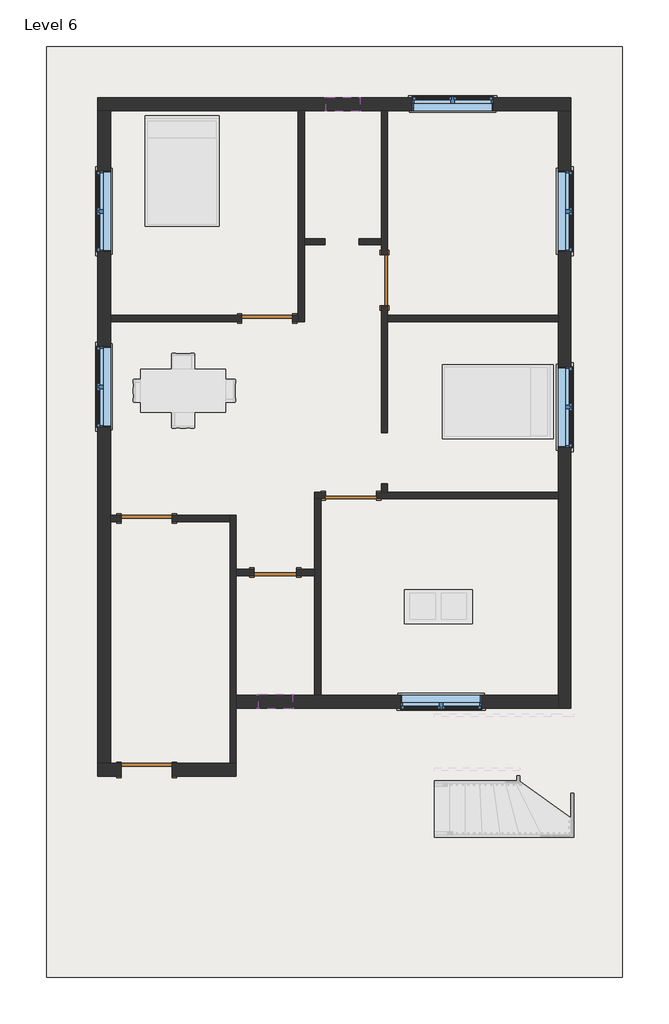
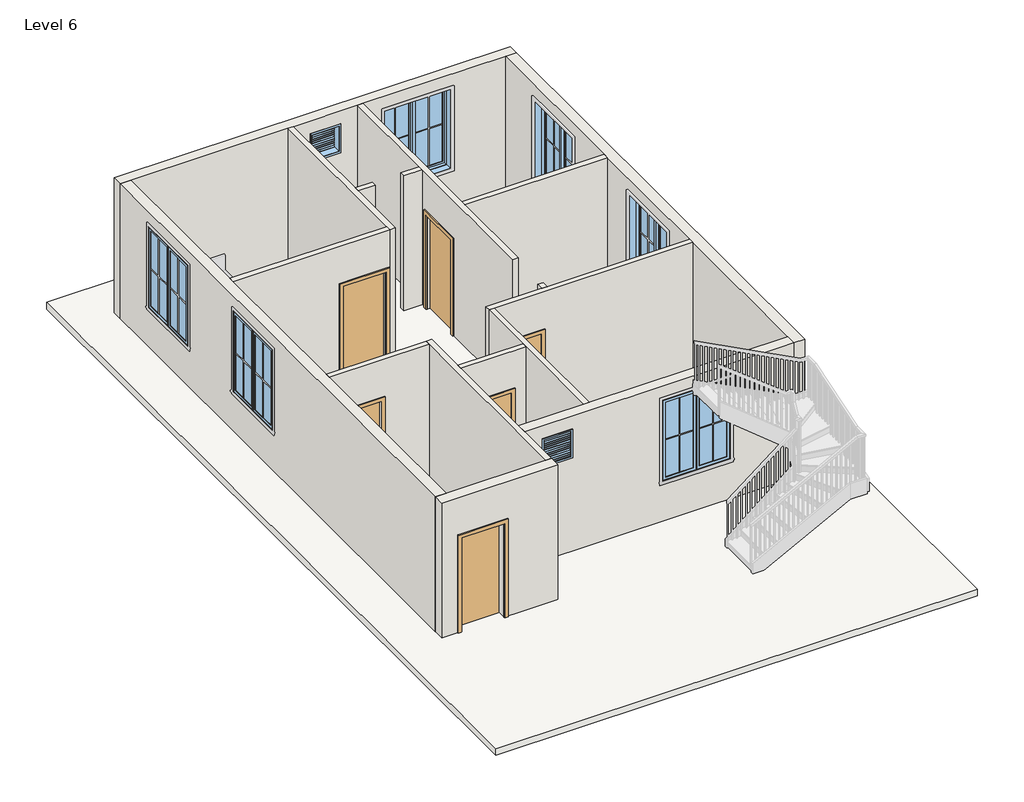
# One storey, part 1 of 3: 17 walls, 8 windows, 6 doors, 1 roof.
"""IFC4 building model written with IfcOpenShell, lengths in millimetres."""

from ifc_helpers import new_model, si_unit, frame, origin, place, context, project, spatial, polyline, outline, extrude, faceted_brep, transform, mapped, element, save
from components import door_214872d5, single_flush_door_3_e5f9f3c4, single_flush_door_3_305aa2a5, single_flush_door_3_a90ba1ad, window_9ac97e1a, window_f2d8fef0

model = new_model("IFC4")

# Units and contexts
model_context = context("Model", 3, world=origin())
ifc_project = project(units=[si_unit("LENGTHUNIT", "METRE", prefix="MILLI")], contexts=[model_context])

# Site, building, storey
site = spatial("IfcSite", under=ifc_project)
building = spatial("IfcBuilding", under=site)
storey = spatial("IfcBuildingStorey", under=building, Name="Level 6", Elevation=12801.6)

# Doors
placement = place(None, origin())
door_shape = door_214872d5(model_context)
element("IfcDoor", 1, ObjectType="Single-Flush : DOOR 2'6\"", at=placement, inside=storey, context=model_context, shape_type="MappedRepresentation", body=[
    mapped(door_shape, transform((-2309.3144966, -2885.2590409, 12801.6), x_axis=(-1.0, 0.0, 0.0), y_axis=(0.0, -1.0, 0.0), z_axis=(0.0, 0.0, 1.0))),
])
single_flush_door_3_shape = single_flush_door_3_e5f9f3c4(model_context)
element("IfcDoor", 2, ObjectType="Single-Flush : DOOR 3'", at=placement, inside=storey, context=model_context, shape_type="MappedRepresentation", body=[
    mapped(single_flush_door_3_shape, transform((-2455.3644966, 1648.6409591, 12801.6), x_axis=(1.0, 0.0, 0.0), y_axis=(0.0, 1.0, 0.0), z_axis=(0.0, 0.0, 1.0))),
])
element("IfcDoor", 3, ObjectType="Single-Flush : DOOR 3'", at=placement, inside=storey, context=model_context, shape_type="MappedRepresentation", body=[
    mapped(single_flush_door_3_shape, transform((-359.8644966, 2334.4409591, 12801.6), x_axis=(0.0, -1.0, 0.0), y_axis=(1.0, 0.0, 0.0), z_axis=(0.0, 0.0, 1.0))),
])
element("IfcDoor", 4, ObjectType="Single-Flush : DOOR 3'", at=placement, inside=storey, context=model_context, shape_type="MappedRepresentation", body=[
    mapped(single_flush_door_3_shape, transform((-956.7644966, -1513.6590409, 12801.6), x_axis=(-1.0, 0.0, 0.0), y_axis=(0.0, -1.0, 0.0), z_axis=(0.0, 0.0, 1.0))),
])
single_flush_door_3_2_shape = single_flush_door_3_305aa2a5(model_context)
element("IfcDoor", 5, ObjectType="Single-Flush : DOOR 3'", at=placement, inside=storey, context=model_context, shape_type="MappedRepresentation", body=[
    mapped(single_flush_door_3_2_shape, transform((-4608.0144966, -1920.0590409, 12801.6), x_axis=(-1.0, 0.0, 0.0), y_axis=(0.0, -1.0, 0.0), z_axis=(0.0, 0.0, 1.0))),
])
single_flush_door_3_3_shape = single_flush_door_3_a90ba1ad(model_context)
element("IfcDoor", 6, ObjectType="Single-Flush : DOOR 3'", at=placement, inside=storey, context=model_context, shape_type="MappedRepresentation", body=[
    mapped(single_flush_door_3_3_shape, transform((-4608.0144966, -6409.5090409, 12801.6), x_axis=(-1.0, 0.0, 0.0), y_axis=(0.0, -1.0, 0.0), z_axis=(0.0, 0.0, 1.0))),
])

# Roof
element("IfcRoof", 7, ObjectType="ROOF 6\"", at=placement, inside=storey, context=model_context, shape_type="SweptSolid", body=[
    extrude(outline(polyline([(-6398.7144966, 6506.3909591), (3888.2855034, 6506.3909591), (3888.2855034, -10115.6142473), (-6398.7144966, -10115.6142473), (-6398.7144966, 6506.3909591)])), frame((0.0, 0.0, 12649.2), z_axis=(0.0, 0.0, 1.0), x_axis=(1.0, 0.0, 0.0)), (0.0, 0.0, 1.0), 152.4),
])

# Walls
element("IfcWall", 8, ObjectType="WALL 4.5\"", at=placement, inside=storey, context=model_context, shape_type="Brep", body=[
    faceted_brep([(-1902.9144966, 5363.3909591, 12801.6), (-1902.9144966, 1705.7909591, 12801.6), (-1902.9144966, 1591.4909591, 12801.6), (-1902.9144966, 1591.4909591, 15849.6), (-1902.9144966, 1705.7909591, 15849.6), (-1902.9144966, 5363.3909591, 15849.6), (-1788.6144966, 5363.3909591, 12801.6), (-1788.6144966, 5363.3909591, 15849.6), (-1788.6144966, 3077.3909591, 15849.6), (-1788.6144966, 2963.0909591, 15849.6), (-1788.6144966, 1591.4909591, 15849.6), (-1788.6144966, 1591.4909591, 12801.6), (-1788.6144966, 2963.0909591, 12801.6), (-1788.6144966, 3077.3909591, 12801.6)], [[[0, 1, 2, 3, 4, 5]], [[6, 7, 8, 9, 10, 11, 12, 13]], [[2, 1, 0, 6, 13, 12, 11]], [[0, 5, 7, 6]], [[3, 2, 11, 10]], [[5, 4, 3, 10, 9, 8, 7]]]),
])
element("IfcWall", 9, ObjectType="WALL 4.5\"", at=placement, inside=storey, context=model_context, shape_type="SweptSolid", body=[
    extrude(outline(polyline([(14935.2, -1998.1644966), (12801.6, -1998.1644966), (12801.6, -1902.9144966), (15849.6, -1902.9144966), (15849.6, -5255.7144966), (12801.6, -5255.7144966), (12801.6, -2912.5644966), (14935.2, -2912.5644966), (14935.2, -1998.1644966)])), frame((0.0, 1591.4909591, 0.0), z_axis=(0.0, 1.0, 0.0), x_axis=(0.0, 0.0, 1.0)), (0.0, 0.0, 1.0), 114.3),
])
element("IfcWall", 10, ObjectType="WALL 4.5\"", at=placement, inside=storey, context=model_context, shape_type="Brep", body=[
    faceted_brep([(-417.0144966, 1877.2409591, 14935.2), (-417.0144966, 1877.2409591, 12801.6), (-417.0144966, -389.7090409, 12801.6), (-417.0144966, -389.7090409, 15849.6), (-417.0144966, 2963.0909591, 15849.6), (-417.0144966, 3077.3909591, 15849.6), (-417.0144966, 5363.3909591, 15849.6), (-417.0144966, 5363.3909591, 12801.6), (-417.0144966, 3077.3909591, 12801.6), (-417.0144966, 2963.0909591, 12801.6), (-417.0144966, 2791.6409591, 12801.6), (-417.0144966, 2791.6409591, 14935.2), (-302.7144966, -389.7090409, 12801.6), (-302.7144966, 1591.4909591, 12801.6), (-302.7144966, 1705.7909591, 12801.6), (-302.7144966, 1877.2409591, 12801.6), (-302.7144966, 1877.2409591, 14935.2), (-302.7144966, 2791.6409591, 14935.2), (-302.7144966, 2791.6409591, 12801.6), (-302.7144966, 5363.3909591, 12801.6), (-302.7144966, 5363.3909591, 15849.6), (-302.7144966, 1705.7909591, 15849.6), (-302.7144966, 1591.4909591, 15849.6), (-302.7144966, -389.7090409, 15849.6)], [[[0, 1, 2, 3, 4, 5, 6, 7, 8, 9, 10, 11]], [[12, 13, 14, 15, 16, 17, 18, 19, 20, 21, 22, 23]], [[2, 1, 15, 14, 13, 12]], [[10, 9, 8, 7, 19, 18]], [[3, 2, 12, 23]], [[7, 6, 20, 19]], [[16, 15, 1, 0]], [[17, 16, 0, 11]], [[18, 17, 11, 10]], [[6, 5, 4, 3, 23, 22, 21, 20]]]),
])
element("IfcWall", 11, ObjectType="WALL 4.5\"", at=placement, inside=storey, context=model_context, shape_type="SweptSolid", body=[
    extrude(outline(polyline([(-302.7144966, 1705.7909591), (2745.2855034, 1705.7909591), (2745.2855034, 1591.4909591), (-302.7144966, 1591.4909591), (-302.7144966, 1705.7909591)])), frame((0.0, 0.0, 12801.6), z_axis=(0.0, 0.0, 1.0), x_axis=(1.0, 0.0, 0.0)), (0.0, 0.0, 1.0), 3048.0),
])
element("IfcWall", 12, ObjectType="WALL 4.5\"", at=placement, inside=storey, context=model_context, shape_type="SweptSolid", body=[
    extrude(outline(polyline([(-1423.1234474, 2963.0909591), (-1788.6144966, 2963.0909591), (-1788.6144966, 3077.3909591), (-1423.1234474, 3077.3909591), (-1423.1234474, 2963.0909591)])), frame((0.0, 0.0, 12801.6), z_axis=(0.0, 0.0, 1.0), x_axis=(1.0, 0.0, 0.0)), (0.0, 0.0, 1.0), 3048.0),
])
element("IfcWall", 13, ObjectType="WALL 4.5\"", at=placement, inside=storey, context=model_context, shape_type="Brep", body=[
    faceted_brep([(-1413.9644966, -1456.5090409, 14935.2), (-1413.9644966, -1456.5090409, 12801.6), (-1610.8144966, -1456.5090409, 12801.6), (-1610.8144966, -1456.5090409, 15849.6), (-417.0144966, -1456.5090409, 15849.6), (-302.7144966, -1456.5090409, 15849.6), (2745.2855034, -1456.5090409, 15849.6), (2745.2855034, -1456.5090409, 12801.6), (-302.7144966, -1456.5090409, 12801.6), (-417.0144966, -1456.5090409, 12801.6), (-499.5644966, -1456.5090409, 12801.6), (-499.5644966, -1456.5090409, 14935.2), (-1610.8144966, -1570.8090409, 12801.6), (-1496.5144966, -1570.8090409, 12801.6), (-1413.9644966, -1570.8090409, 12801.6), (-1413.9644966, -1570.8090409, 14935.2), (-499.5644966, -1570.8090409, 14935.2), (-499.5644966, -1570.8090409, 12801.6), (2745.2855034, -1570.8090409, 12801.6), (2745.2855034, -1570.8090409, 15849.6), (-1496.5144966, -1570.8090409, 15849.6), (-1610.8144966, -1570.8090409, 15849.6)], [[[0, 1, 2, 3, 4, 5, 6, 7, 8, 9, 10, 11]], [[12, 13, 14, 15, 16, 17, 18, 19, 20, 21]], [[2, 1, 14, 13, 12]], [[10, 9, 8, 7, 18, 17]], [[7, 6, 19, 18]], [[3, 2, 12, 21]], [[15, 14, 1, 0]], [[16, 15, 0, 11]], [[17, 16, 11, 10]], [[6, 5, 4, 3, 21, 20, 19]]]),
])
element("IfcWall", 14, ObjectType="WALL 4.5\"", at=placement, inside=storey, context=model_context, shape_type="SweptSolid", body=[
    extrude(outline(polyline([(-302.7144966, -1304.1090409), (-302.7144966, -1456.5090409), (-417.0144966, -1456.5090409), (-417.0144966, -1304.1090409), (-302.7144966, -1304.1090409)])), frame((0.0, 0.0, 12801.6), z_axis=(0.0, 0.0, 1.0), x_axis=(1.0, 0.0, 0.0)), (0.0, 0.0, 1.0), 3048.0),
])
element("IfcWall", 15, ObjectType="WALL 4.5\"", at=placement, inside=storey, context=model_context, shape_type="Brep", body=[
    faceted_brep([(-1610.8144966, -1570.8090409, 12801.6), (-1610.8144966, -2828.1090409, 12801.6), (-1610.8144966, -2942.4090409, 12801.6), (-1610.8144966, -5076.0090409, 12801.6), (-1610.8144966, -5076.0090409, 15849.6), (-1610.8144966, -2942.4090409, 15849.6), (-1610.8144966, -2828.1090409, 15849.6), (-1610.8144966, -1570.8090409, 15849.6), (-1496.5144966, -1570.8090409, 12801.6), (-1496.5144966, -1570.8090409, 15849.6), (-1496.5144966, -5076.0090409, 15849.6), (-1496.5144966, -5076.0090409, 12801.6)], [[[0, 1, 2, 3, 4, 5, 6, 7]], [[8, 9, 10, 11]], [[3, 2, 1, 0, 8, 11]], [[0, 7, 9, 8]], [[4, 3, 11, 10]], [[7, 6, 5, 4, 10, 9]]]),
])
element("IfcWall", 16, ObjectType="WALL 4.5\"", at=placement, inside=storey, context=model_context, shape_type="SweptSolid", body=[
    extrude(outline(polyline([(12801.6, -3007.8144966), (12801.6, -2690.3144966), (14935.2, -2690.3144966), (14935.2, -1928.3144966), (12801.6, -1928.3144966), (12801.6, -1610.8144966), (15849.6, -1610.8144966), (15849.6, -3007.8144966), (12801.6, -3007.8144966)])), frame((0.0, -2942.4090409, 0.0), z_axis=(0.0, 1.0, 0.0), x_axis=(0.0, 0.0, 1.0)), (0.0, 0.0, 1.0), 114.3),
])
element("IfcWall", 17, ObjectType="WALL 4.5\"", at=placement, inside=storey, context=model_context, shape_type="Brep", body=[
    faceted_brep([(-3007.8144966, -6295.2090409, 12801.6), (-3007.8144966, -5304.6090409, 12801.6), (-3007.8144966, -5076.0090409, 12801.6), (-3007.8144966, -2942.4090409, 12801.6), (-3007.8144966, -2828.1090409, 12801.6), (-3007.8144966, -1862.9090409, 12801.6), (-3007.8144966, -1862.9090409, 15849.6), (-3007.8144966, -2828.1090409, 15849.6), (-3007.8144966, -2942.4090409, 15849.6), (-3007.8144966, -5076.0090409, 15849.6), (-3007.8144966, -5304.6090409, 15849.6), (-3007.8144966, -6295.2090409, 15849.6), (-3122.1144966, -6295.2090409, 12801.6), (-3122.1144966, -6295.2090409, 15849.6), (-3122.1144966, -1977.2090409, 15849.6), (-3122.1144966, -1862.9090409, 15849.6), (-3122.1144966, -1862.9090409, 12801.6), (-3122.1144966, -1977.2090409, 12801.6)], [[[0, 1, 2, 3, 4, 5, 6, 7, 8, 9, 10, 11]], [[12, 13, 14, 15, 16, 17]], [[5, 4, 3, 2, 1, 0, 12, 17, 16]], [[0, 11, 13, 12]], [[6, 5, 16, 15]], [[11, 10, 9, 8, 7, 6, 15, 14, 13]]]),
])
element("IfcWall", 18, ObjectType="WALL 4.5\"", at=placement, inside=storey, context=model_context, shape_type="SweptSolid", body=[
    extrude(outline(polyline([(12801.6, -5255.7144966), (12801.6, -5065.2144966), (14935.2, -5065.2144966), (14935.2, -4150.8144966), (12801.6, -4150.8144966), (12801.6, -3122.1144966), (15849.6, -3122.1144966), (15849.6, -5255.7144966), (12801.6, -5255.7144966)])), frame((0.0, -1977.2090409, 0.0), z_axis=(0.0, 1.0, 0.0), x_axis=(0.0, 0.0, 1.0)), (0.0, 0.0, 1.0), 114.3),
])
element("IfcWall", 19, ObjectType="WALL 4.5\"", at=placement, inside=storey, context=model_context, shape_type="SweptSolid", body=[
    extrude(outline(polyline([(-417.0144966, 2963.0909591), (-814.3659123, 2963.0909591), (-814.3659123, 3077.3909591), (-417.0144966, 3077.3909591), (-417.0144966, 2963.0909591)])), frame((0.0, 0.0, 12801.6), z_axis=(0.0, 0.0, 1.0), x_axis=(1.0, 0.0, 0.0)), (0.0, 0.0, 1.0), 3048.0),
])
element("IfcWall", 20, ObjectType="WALL 9\"", at=placement, inside=storey, context=model_context, shape_type="Brep", body=[
    faceted_brep([(-5484.3144966, 5363.3909591, 12801.6), (-5255.7144966, 5363.3909591, 12801.6), (-1902.9144966, 5363.3909591, 12801.6), (-1788.6144966, 5363.3909591, 12801.6), (-417.0144966, 5363.3909591, 12801.6), (-302.7144966, 5363.3909591, 12801.6), (2745.2855034, 5363.3909591, 12801.6), (2973.8855034, 5363.3909591, 12801.6), (2973.8855034, 5363.3909591, 15849.6), (2745.2855034, 5363.3909591, 15849.6), (-302.7144966, 5363.3909591, 15849.6), (-417.0144966, 5363.3909591, 15849.6), (-1788.6144966, 5363.3909591, 15849.6), (-1902.9144966, 5363.3909591, 15849.6), (-5255.7144966, 5363.3909591, 15849.6), (-5484.3144966, 5363.3909591, 15849.6), (1583.2355034, 5363.3909591, 15544.8), (1583.2355034, 5363.3909591, 13716.0), (135.4355034, 5363.3909591, 13716.0), (135.4355034, 5363.3909591, 15544.8), (-1407.6144966, 5363.3909591, 15544.8), (-798.0144966, 5363.3909591, 15544.8), (-798.0144966, 5363.3909591, 14935.2), (-1407.6144966, 5363.3909591, 14935.2), (-5484.3144966, 5591.9909591, 12801.6), (-5484.3144966, 5591.9909591, 15849.6), (2973.8855034, 5591.9909591, 15849.6), (2973.8855034, 5591.9909591, 12801.6), (1583.2355034, 5591.9909591, 15544.8), (135.4355034, 5591.9909591, 15544.8), (135.4355034, 5591.9909591, 13716.0), (1583.2355034, 5591.9909591, 13716.0), (-1407.6144966, 5591.9909591, 15544.8), (-1407.6144966, 5591.9909591, 14935.2), (-798.0144966, 5591.9909591, 14935.2), (-798.0144966, 5591.9909591, 15544.8)], [[[0, 1, 2, 3, 4, 5, 6, 7, 8, 9, 10, 11, 12, 13, 14, 15], [16, 17, 18, 19], [20, 21, 22, 23]], [[24, 25, 26, 27], [28, 29, 30, 31], [32, 33, 34, 35]], [[7, 6, 5, 4, 3, 2, 1, 0, 24, 27]], [[8, 7, 27, 26]], [[0, 15, 25, 24]], [[17, 16, 28, 31]], [[18, 17, 31, 30]], [[19, 18, 30, 29]], [[16, 19, 29, 28]], [[33, 32, 20, 23]], [[34, 33, 23, 22]], [[35, 34, 22, 21]], [[32, 35, 21, 20]], [[15, 14, 13, 12, 11, 10, 9, 8, 26, 25]]]),
])
element("IfcWall", 21, ObjectType="WALL 9\"", at=placement, inside=storey, context=model_context, shape_type="Brep", body=[
    faceted_brep([(2745.2855034, 5363.3909591, 12801.6), (2745.2855034, 1705.7909591, 12801.6), (2745.2855034, 1591.4909591, 12801.6), (2745.2855034, -1456.5090409, 12801.6), (2745.2855034, -1570.8090409, 12801.6), (2745.2855034, -5076.0090409, 12801.6), (2745.2855034, -5304.6090409, 12801.6), (2745.2855034, -5304.6090409, 15849.6), (2745.2855034, -5076.0090409, 15849.6), (2745.2855034, -1570.8090409, 15849.6), (2745.2855034, -1456.5090409, 15849.6), (2745.2855034, 1591.4909591, 15849.6), (2745.2855034, 1705.7909591, 15849.6), (2745.2855034, 5363.3909591, 15849.6), (2745.2855034, -656.4090409, 15544.8), (2745.2855034, -656.4090409, 13716.0), (2745.2855034, 791.3909591, 13716.0), (2745.2855034, 791.3909591, 15544.8), (2745.2855034, 2839.2659591, 15544.8), (2745.2855034, 2839.2659591, 13716.0), (2745.2855034, 4287.0659591, 13716.0), (2745.2855034, 4287.0659591, 15544.8), (2973.8855034, 5363.3909591, 12801.6), (2973.8855034, 5363.3909591, 15849.6), (2973.8855034, -5304.6090409, 15849.6), (2973.8855034, -5304.6090409, 12801.6), (2973.8855034, -656.4090409, 15544.8), (2973.8855034, 791.3909591, 15544.8), (2973.8855034, 791.3909591, 13716.0), (2973.8855034, -656.4090409, 13716.0), (2973.8855034, 2839.2659591, 15544.8), (2973.8855034, 4287.0659591, 15544.8), (2973.8855034, 4287.0659591, 13716.0), (2973.8855034, 2839.2659591, 13716.0)], [[[0, 1, 2, 3, 4, 5, 6, 7, 8, 9, 10, 11, 12, 13], [14, 15, 16, 17], [18, 19, 20, 21]], [[22, 23, 24, 25], [26, 27, 28, 29], [30, 31, 32, 33]], [[6, 5, 4, 3, 2, 1, 0, 22, 25]], [[0, 13, 23, 22]], [[7, 6, 25, 24]], [[15, 14, 26, 29]], [[16, 15, 29, 28]], [[17, 16, 28, 27]], [[14, 17, 27, 26]], [[19, 18, 30, 33]], [[20, 19, 33, 32]], [[21, 20, 32, 31]], [[18, 21, 31, 30]], [[13, 12, 11, 10, 9, 8, 7, 24, 23]]]),
])
element("IfcWall", 22, ObjectType="WALL 9\"", at=placement, inside=storey, context=model_context, shape_type="Brep", body=[
    faceted_brep([(2745.2855034, -5076.0090409, 12801.6), (-1496.5144966, -5076.0090409, 12801.6), (-1610.8144966, -5076.0090409, 12801.6), (-3007.8144966, -5076.0090409, 12801.6), (-3007.8144966, -5076.0090409, 15849.6), (-1610.8144966, -5076.0090409, 15849.6), (-1496.5144966, -5076.0090409, 15849.6), (2745.2855034, -5076.0090409, 15849.6), (-70.9394966, -5076.0090409, 15544.8), (-70.9394966, -5076.0090409, 13716.0), (1376.8605034, -5076.0090409, 13716.0), (1376.8605034, -5076.0090409, 15544.8), (-2004.5144966, -5076.0090409, 15544.8), (-2614.1144966, -5076.0090409, 15544.8), (-2614.1144966, -5076.0090409, 14935.2), (-2004.5144966, -5076.0090409, 14935.2), (2745.2855034, -5304.6090409, 12801.6), (2745.2855034, -5304.6090409, 15849.6), (-3007.8144966, -5304.6090409, 15849.6), (-3007.8144966, -5304.6090409, 12801.6), (-70.9394966, -5304.6090409, 15544.8), (1376.8605034, -5304.6090409, 15544.8), (1376.8605034, -5304.6090409, 13716.0), (-70.9394966, -5304.6090409, 13716.0), (-2004.5144966, -5304.6090409, 15544.8), (-2004.5144966, -5304.6090409, 14935.2), (-2614.1144966, -5304.6090409, 14935.2), (-2614.1144966, -5304.6090409, 15544.8)], [[[0, 1, 2, 3, 4, 5, 6, 7], [8, 9, 10, 11], [12, 13, 14, 15]], [[16, 17, 18, 19], [20, 21, 22, 23], [24, 25, 26, 27]], [[3, 2, 1, 0, 16, 19]], [[0, 7, 17, 16]], [[4, 3, 19, 18]], [[9, 8, 20, 23]], [[10, 9, 23, 22]], [[11, 10, 22, 21]], [[8, 11, 21, 20]], [[25, 24, 12, 15]], [[26, 25, 15, 14]], [[27, 26, 14, 13]], [[24, 27, 13, 12]], [[7, 6, 5, 4, 18, 17]]]),
])
element("IfcWall", 23, ObjectType="WALL 9\"", at=placement, inside=storey, context=model_context, shape_type="Brep", body=[
    faceted_brep([(-5065.2144966, -6295.2090409, 14935.2), (-5065.2144966, -6295.2090409, 12801.6), (-5255.7144966, -6295.2090409, 12801.6), (-5484.3144966, -6295.2090409, 12801.6), (-5484.3144966, -6295.2090409, 15849.6), (-5255.7144966, -6295.2090409, 15849.6), (-3122.1144966, -6295.2090409, 15849.6), (-3007.8144966, -6295.2090409, 15849.6), (-3007.8144966, -6295.2090409, 12801.6), (-3122.1144966, -6295.2090409, 12801.6), (-4150.8144966, -6295.2090409, 12801.6), (-4150.8144966, -6295.2090409, 14935.2), (-5484.3144966, -6523.8090409, 12801.6), (-5065.2144966, -6523.8090409, 12801.6), (-5065.2144966, -6523.8090409, 14935.2), (-4150.8144966, -6523.8090409, 14935.2), (-4150.8144966, -6523.8090409, 12801.6), (-3007.8144966, -6523.8090409, 12801.6), (-3007.8144966, -6523.8090409, 15849.6), (-5484.3144966, -6523.8090409, 15849.6)], [[[0, 1, 2, 3, 4, 5, 6, 7, 8, 9, 10, 11]], [[12, 13, 14, 15, 16, 17, 18, 19]], [[10, 9, 8, 17, 16]], [[3, 2, 1, 13, 12]], [[4, 3, 12, 19]], [[8, 7, 18, 17]], [[7, 6, 5, 4, 19, 18]], [[14, 13, 1, 0]], [[15, 14, 0, 11]], [[16, 15, 11, 10]]]),
])
element("IfcWall", 24, ObjectType="WALL 9\"", at=placement, inside=storey, context=model_context, shape_type="Brep", body=[
    faceted_brep([(-5255.7144966, -6295.2090409, 12801.6), (-5255.7144966, -1977.2090409, 12801.6), (-5255.7144966, -1862.9090409, 12801.6), (-5255.7144966, 1591.4909591, 12801.6), (-5255.7144966, 1705.7909591, 12801.6), (-5255.7144966, 5363.3909591, 12801.6), (-5255.7144966, 5363.3909591, 15849.6), (-5255.7144966, 1705.7909591, 15849.6), (-5255.7144966, 1591.4909591, 15849.6), (-5255.7144966, -1862.9090409, 15849.6), (-5255.7144966, -1977.2090409, 15849.6), (-5255.7144966, -6295.2090409, 15849.6), (-5255.7144966, 4287.0659591, 15544.8), (-5255.7144966, 4287.0659591, 13716.0), (-5255.7144966, 2839.2659591, 13716.0), (-5255.7144966, 2839.2659591, 15544.8), (-5255.7144966, 1153.3409591, 15544.8), (-5255.7144966, 1153.3409591, 13716.0), (-5255.7144966, -294.4590409, 13716.0), (-5255.7144966, -294.4590409, 15544.8), (-5484.3144966, -6295.2090409, 12801.6), (-5484.3144966, -6295.2090409, 15849.6), (-5484.3144966, 5363.3909591, 15849.6), (-5484.3144966, 5363.3909591, 12801.6), (-5484.3144966, 4287.0659591, 15544.8), (-5484.3144966, 2839.2659591, 15544.8), (-5484.3144966, 2839.2659591, 13716.0), (-5484.3144966, 4287.0659591, 13716.0), (-5484.3144966, 1153.3409591, 15544.8), (-5484.3144966, -294.4590409, 15544.8), (-5484.3144966, -294.4590409, 13716.0), (-5484.3144966, 1153.3409591, 13716.0)], [[[0, 1, 2, 3, 4, 5, 6, 7, 8, 9, 10, 11], [12, 13, 14, 15], [16, 17, 18, 19]], [[20, 21, 22, 23], [24, 25, 26, 27], [28, 29, 30, 31]], [[5, 4, 3, 2, 1, 0, 20, 23]], [[0, 11, 21, 20]], [[6, 5, 23, 22]], [[13, 12, 24, 27]], [[14, 13, 27, 26]], [[15, 14, 26, 25]], [[12, 15, 25, 24]], [[17, 16, 28, 31]], [[18, 17, 31, 30]], [[19, 18, 30, 29]], [[16, 19, 29, 28]], [[11, 10, 9, 8, 7, 6, 22, 21]]]),
])

# Windows
window_shape = window_9ac97e1a(model_context)
element("IfcWindow", 25, ObjectType="Window-Casement-Double : 57\" x 72\"", at=placement, inside=storey, context=model_context, shape_type="MappedRepresentation", body=[
    mapped(window_shape, transform((2859.5855034, 67.4909591, 12801.6), x_axis=(0.0, -1.0, 0.0), y_axis=(1.0, 0.0, 0.0), z_axis=(0.0, 0.0, 1.0))),
])
element("IfcWindow", 26, ObjectType="Window-Casement-Double : 57\" x 72\"", at=placement, inside=storey, context=model_context, shape_type="MappedRepresentation", body=[
    mapped(window_shape, transform((2859.5855034, 3563.1659591, 12801.6), x_axis=(0.0, -1.0, 0.0), y_axis=(1.0, 0.0, 0.0), z_axis=(0.0, 0.0, 1.0))),
])
element("IfcWindow", 27, ObjectType="Window-Casement-Double : 57\" x 72\"", at=placement, inside=storey, context=model_context, shape_type="MappedRepresentation", body=[
    mapped(window_shape, transform((859.3355034, 5477.6909591, 12801.6), x_axis=(1.0, 0.0, 0.0), y_axis=(0.0, 1.0, 0.0), z_axis=(0.0, 0.0, 1.0))),
])
element("IfcWindow", 28, ObjectType="Window-Casement-Double : 57\" x 72\"", at=placement, inside=storey, context=model_context, shape_type="MappedRepresentation", body=[
    mapped(window_shape, transform((-5370.0144966, 3563.1659591, 12801.6), x_axis=(0.0, 1.0, 0.0), y_axis=(-1.0, 0.0, 0.0), z_axis=(0.0, 0.0, 1.0))),
])
element("IfcWindow", 29, ObjectType="Window-Casement-Double : 57\" x 72\"", at=placement, inside=storey, context=model_context, shape_type="MappedRepresentation", body=[
    mapped(window_shape, transform((-5370.0144966, 429.4409591, 12801.6), x_axis=(0.0, 1.0, 0.0), y_axis=(-1.0, 0.0, 0.0), z_axis=(0.0, 0.0, 1.0))),
])
element("IfcWindow", 30, ObjectType="Window-Casement-Double : 57\" x 72\"", at=placement, inside=storey, context=model_context, shape_type="MappedRepresentation", body=[
    mapped(window_shape, transform((652.9605034, -5190.3090409, 12801.6), x_axis=(-1.0, 0.0, 0.0), y_axis=(0.0, -1.0, 0.0), z_axis=(0.0, 0.0, 1.0))),
])
window_2_shape = window_f2d8fef0(model_context)
element("IfcWindow", 31, ObjectType="Window-Louvers : 24\" x 24\"", at=placement, inside=storey, context=model_context, shape_type="MappedRepresentation", body=[
    mapped(window_2_shape, transform((-1102.8144966, 5484.0409591, 14020.8), x_axis=(1.0, 0.0, 0.0), y_axis=(0.0, 1.0, 0.0), z_axis=(0.0, 0.0, 1.0))),
])
element("IfcWindow", 32, ObjectType="Window-Louvers : 24\" x 24\"", at=placement, inside=storey, context=model_context, shape_type="MappedRepresentation", body=[
    mapped(window_2_shape, transform((-2309.3144966, -5196.6590409, 14020.8), x_axis=(-1.0, 0.0, 0.0), y_axis=(0.0, -1.0, 0.0), z_axis=(0.0, 0.0, 1.0))),
])

save(model, "model.ifc")

# Revit data of these elements
# Type "Single-Flush : DOOR 2'6\""
#   Type Mark = "10"
#   Construction Type Id = "MDOOR"
#   Assembly Code = "C1020"
#   Analytic Construction = "Metal"
#   Thickness = 0' - 2"
#   Heat Transfer Coefficient (U) = 0.651978 BTU/(h·ft²·°F)
#   Height = 7' - 0"
#   Trim Projection Ext = 0' - 1"
#   Trim Projection Int = 0' - 1"
#   Trim Width = 0' - 3"
#   Width = 2' - 6"
#   Define Thermal Properties by = 1
#   Door Material = Door - Panel
#   Frame Material = Door - Frame
#   Visual Light Transmittance = 0
#   Solar Heat Gain Coefficient = 0
#   Function = (empty or 0)
#   Wall Closure = (empty or 0)
# Type "Single-Flush : DOOR 3'"
#   Type Mark = "9"
#   Construction Type Id = "MDOOR"
#   Assembly Code = "C1020"
#   Analytic Construction = "Metal"
#   Thickness = 0' - 2"
#   Heat Transfer Coefficient (U) = 0.651978 BTU/(h·ft²·°F)
#   Height = 7' - 0"
#   Trim Projection Ext = 0' - 1"
#   Trim Projection Int = 0' - 1"
#   Trim Width = 0' - 3"
#   Width = 3' - 0"
#   Define Thermal Properties by = 1
#   Door Material = Door - Panel
#   Frame Material = Door - Frame
#   Visual Light Transmittance = 0
#   Solar Heat Gain Coefficient = 0
#   Function = (empty or 0)
#   Wall Closure = (empty or 0)
# Type "ROOF 6\""
#   Assembly Code = "B1020"
#   Layers, outside or top first: 0' - 6" no material (function 1)
# Type "WALL 4.5\""
#   Assembly Code = "B2010"
#   Layers, outside or top first: 0' - 4 1/2" no material (function 1)
# Type "WALL 9\""
#   Assembly Code = "B2010"
#   Layers, outside or top first: 0' - 9" no material (function 1)
# Type "Window-Casement-Double : 57\" x 72\""
#   Type Mark = "17"
#   Fire Rating = "0.5h"
#   Assembly Code = "B2020100"
#   Analytic Construction = "Double glazing - domestic"
#   Frame Extension [instance default] = 0' - 0 1/4"
#   Window Inset [instance default] = 0' - 0"
#   Wall Thickness [instance default] = 0' - 6"
#   Interior Wall Closure [instance default] = 0' - 2 1/4"
#   Half Width = 2' - 4 1/2"
#   Visual Light Transmittance = 0.81
#   Thermal Resistance (R) = 1.8146 (h·ft²·°F)/BTU
#   Solar Heat Gain Coefficient = 0.76
#   Rough Width = 4' - 9 1/2"
#   Rough Height = 6' - 0 1/2"
#   Height = 6' - 0"
#   Heat Transfer Coefficient (U) = 0.5511 BTU/(h·ft²·°F)
#   Exterior Wall Closure [instance default] = 0' - 1 1/4"
#   Extension Jamb [instance default] = 0' - 2 1/4"
#   Default Sill Height = 3' - 0"
#   Width = 4' - 9"
#   Define Thermal Properties by = 0
#   Muntin Visibility = yes
#   Interior Trim Visibility [instance default] = yes
#   Exterior Trim Visibility [instance default] = yes
#   Extension Jamb Visibility [instance default] = yes
#   Interior Trim Material = Wood - Stained
#   Muntin Pattern = Muntin Pattern_2x2 : Muntin Pattern_2x2
#   Interior Trim = Trim-Window-Interior-Flat : Picture Frame
#   Interior Frame Material = Wood - Stained
#   Glass Panel Material = Glass
#   Exterior Trim Material = Clad - White
#   Exterior Trim = Trim-Window-Exterior-Flat : with Sill
#   Exterior Frame Material = Clad - White
#   Wall Closure = (empty or 0)
# Type "Window-Louvers : 24\" x 24\""
#   Type Mark = "18"
#   Construction Type Id = "GSP4R"
#   Assembly Code = "B20"
#   Analytic Construction = "1/8 in Pilkington single glazing"
#   Visual Light Transmittance = 0.9
#   Thermal Resistance (R) = 1.53941 (h·ft²·°F)/BTU
#   Solar Heat Gain Coefficient = 0.78
#   Max Height = 1' - 11.74264"
#   Height = 2' - 0"
#   Heat Transfer Coefficient (U) = 0.6496 BTU/(h·ft²·°F)
#   Blade Width [instance default] = 1' - 10 1/2"
#   Blade Vertical Thickness = 0' - 0.35355"
#   Blade Thickness = 0' - 0 1/4"
#   Blade Spacing = 0' - 1 1/2"
#   Blade Height = 0' - 1.85355"
#   Blade Depth = 0' - 3"
#   Blade Angle = 45.00°
#   Default Sill Height = 3' - 0"
#   Trim Projection_Exterior = 0' - 0 1/2"
#   Trim Projection_Interior = 0' - 0 1/2"
#   Trim Width_Exterior = 0' - 1 1/2"
#   Trim Width_Interior = 0' - 1 1/2"
#   Width = 2' - 0"
#   Max Blade Count = 12
#   Define Thermal Properties by = 1
#   Blade Count = 12
#   Frame Material = Birch
#   Louver Material = Birch
#   Trim Exterior Material = Birch
#   Trim Interior Material = Birch
#   Wall Closure = (empty or 0)
# Element 1 (IfcDoor, "Single-Flush : DOOR 2'6\"")
#   Phase Created = New Construction
#   Materials on its faces: "Door - Frame", "Door - Panel"
# Elements 2, 3, 4, 5, 6 (IfcDoor, "Single-Flush : DOOR 3'")
#   Phase Created = New Construction
#   Materials on its faces: "Door - Frame", "Door - Panel"
# Element 7 (IfcRoof, "ROOF 6\"")
#   built-in parameter 1001705 = 42 (stored number, unit not read)
#   built-in parameter 1001701 = -0.5 (stored number, unit not read)
#   built-in parameter 1001710 = 33615
#   Phase Created = New Construction
#   Materials on its faces: "Cherry", "Default Roof", "Softwood, Lumber"
# Elements 8, 9, 10, 11, 12, 13, 14, 15, 16, 17, 18, 19 (IfcWall, "WALL 4.5\"")
#   Top Offset = 0' - 0"
#   Base Offset = 0' - 0"
#   Unconnected Height = 10' - 0"
#   wall height = 10' - 0"
#   Phase Created = New Construction
#   Base Constraint = Level 6
#   Materials on its faces: "Default Wall"
# Elements 20, 21, 22, 23, 24 (IfcWall, "WALL 9\"")
#   Top Offset = 0' - 0"
#   Base Offset = 0' - 0"
#   Unconnected Height = 10' - 0"
#   wall height = 10' - 0"
#   Phase Created = New Construction
#   Base Constraint = Level 6
#   Materials on its faces: "Default Wall"
# Element 25 (IfcWindow, "Window-Casement-Double : 57\" x 72\"")
#   Mark = "33"
#   Window Inset = 0' - 0"
#   Interior Wall Closure = 0' - 2 1/4"
#   Frame Extension = 0' - 0 1/4"
#   Exterior Wall Closure = 0' - 1 1/4"
#   Interior Trim Visibility = yes
#   Exterior Trim Visibility = yes
#   Phase Created = New Construction
#   Materials on its faces: "Wood - Stained", "Glass", "Clad - White"
# Element 26 (IfcWindow, "Window-Casement-Double : 57\" x 72\"")
#   Mark = "34"
#   Window Inset = 0' - 0"
#   Interior Wall Closure = 0' - 2 1/4"
#   Frame Extension = 0' - 0 1/4"
#   Exterior Wall Closure = 0' - 1 1/4"
#   Interior Trim Visibility = yes
#   Exterior Trim Visibility = yes
#   Phase Created = New Construction
#   Materials on its faces: "Wood - Stained", "Glass", "Clad - White"
# Element 27 (IfcWindow, "Window-Casement-Double : 57\" x 72\"")
#   Mark = "35"
#   Window Inset = 0' - 0"
#   Interior Wall Closure = 0' - 2 1/4"
#   Frame Extension = 0' - 0 1/4"
#   Exterior Wall Closure = 0' - 1 1/4"
#   Interior Trim Visibility = yes
#   Exterior Trim Visibility = yes
#   Phase Created = New Construction
#   Materials on its faces: "Wood - Stained", "Glass", "Clad - White"
# Element 28 (IfcWindow, "Window-Casement-Double : 57\" x 72\"")
#   Mark = "36"
#   Window Inset = 0' - 0"
#   Interior Wall Closure = 0' - 2 1/4"
#   Frame Extension = 0' - 0 1/4"
#   Exterior Wall Closure = 0' - 1 1/4"
#   Interior Trim Visibility = yes
#   Exterior Trim Visibility = yes
#   Phase Created = New Construction
#   Materials on its faces: "Wood - Stained", "Glass", "Clad - White"
# Element 29 (IfcWindow, "Window-Casement-Double : 57\" x 72\"")
#   Mark = "37"
#   Window Inset = 0' - 0"
#   Interior Wall Closure = 0' - 2 1/4"
#   Frame Extension = 0' - 0 1/4"
#   Exterior Wall Closure = 0' - 1 1/4"
#   Interior Trim Visibility = yes
#   Exterior Trim Visibility = yes
#   Phase Created = New Construction
#   Materials on its faces: "Wood - Stained", "Glass", "Clad - White"
# Element 30 (IfcWindow, "Window-Casement-Double : 57\" x 72\"")
#   Mark = "38"
#   Window Inset = 0' - 0"
#   Interior Wall Closure = 0' - 2 1/4"
#   Frame Extension = 0' - 0 1/4"
#   Exterior Wall Closure = 0' - 1 1/4"
#   Interior Trim Visibility = yes
#   Exterior Trim Visibility = yes
#   Phase Created = New Construction
#   Materials on its faces: "Wood - Stained", "Glass", "Clad - White"
# Element 31 (IfcWindow, "Window-Louvers : 24\" x 24\"")
#   Mark = "39"
#   Blade Width = 1' - 10 1/2"
#   Phase Created = New Construction
#   Materials on its faces: "Birch"
# Element 32 (IfcWindow, "Window-Louvers : 24\" x 24\"")
#   Mark = "40"
#   Blade Width = 1' - 10 1/2"
#   Phase Created = New Construction
#   Materials on its faces: "Birch"
# Materials
#   "Door - Panel": class "Wood", colour RGB 210 159 95, transparency 0, Cost = 0
#   "Door - Frame": colour RGB 118 70 51, transparency 0, Cost = 0
#   "Wood - Stained": class "Wood", colour RGB 224 178 126, transparency 0, Cost = 0
#   "Glass": class "Glass", colour RGB 0 128 192, transparency 0.75, Description = "Soda Lime Glass", Cost = 0
#   "Clad - White": class "Wood", colour RGB 242 242 238, transparency 0, Cost = 0
#   "Birch": class "Wood", colour RGB 224 178 126, transparency 0, Description = "Betula Alleghaniensis", Cost = 0
#   "Cherry": class "Wood", colour RGB 226 177 128, transparency 0, Description = "Prunus Serotina", Cost = 0
#   "Default Roof": colour RGB 88 101 114, transparency 0, Cost = 0
#   "Softwood, Lumber": class "Wood", colour RGB 223 192 134, transparency 0, Description = "Pinus Echinata", Cost = 0
#   "Default Wall": colour RGB 128 128 128, transparency 0, Cost = 0
